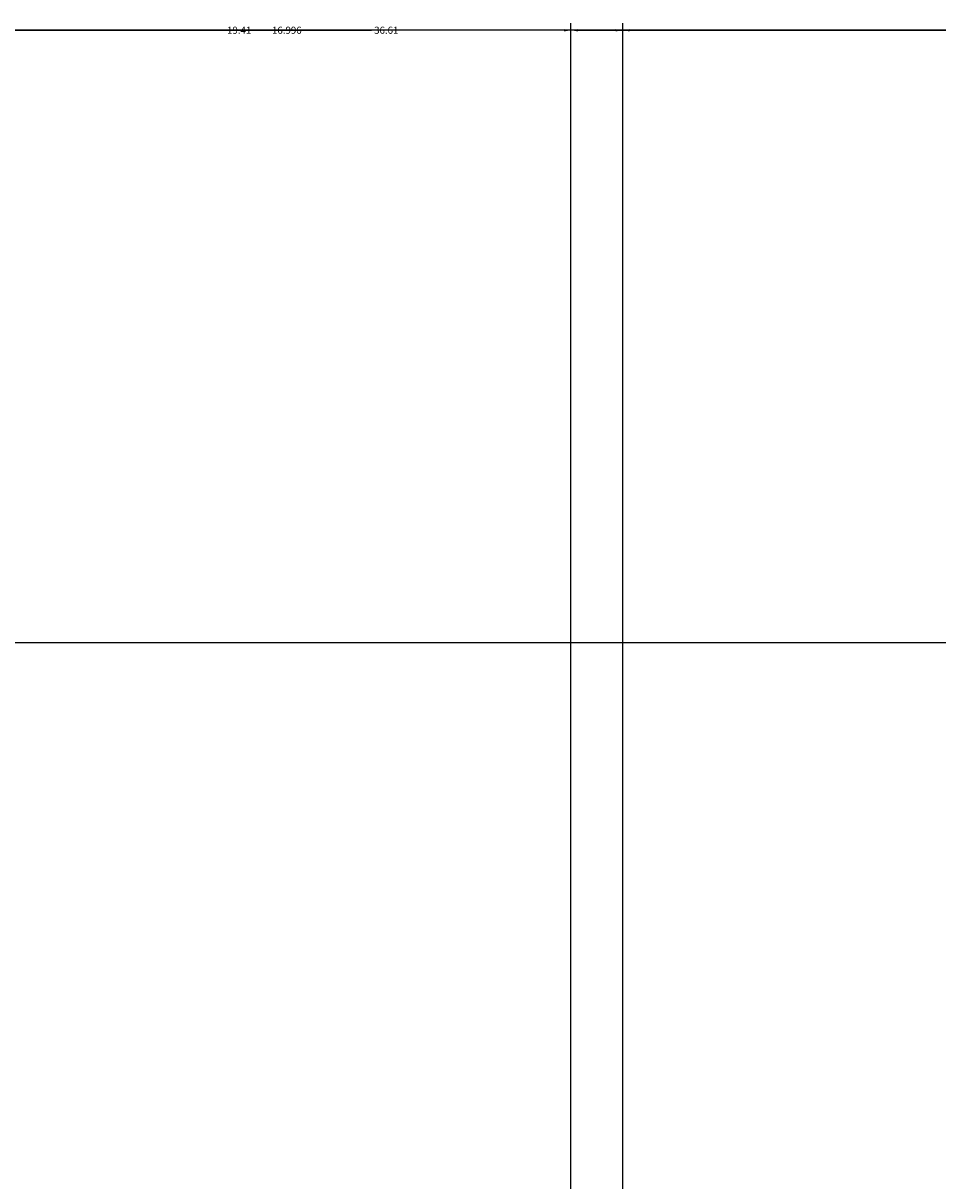
# Model space of a CAD drawing. Units: inches. Extents: x -6 to 289, y -8 to 323.
# Tile 92 of 107: x 173 to 196, y 294 to 323. Entities that reach past the tile are written whole.
import ezdxf

# ---------------------------------------------------------------- set-up
doc = ezdxf.new("R2010")
doc.units = ezdxf.units.IN
doc.header["$MEASUREMENT"] = 0
doc.layers.add('A-ANNO-DIMS', color=2, linetype='Continuous', lineweight=18)
doc.styles.get("Standard").update_dxf_attribs({"font": 'arial.ttf'})
doc.dimstyles.get("Standard").update_dxf_attribs({"dimtxt": 0.18, "dimasz": 0.18, "dimexe": 0.18, "dimexo": 0.0625, "dimgap": 0.09, "dimtad": 0, "dimtih": 1, "dimtoh": 1, "dimdec": 4, "dimzin": 0, "dimdsep": 46, "dimtxsty": 'Standard', "dimcen": 0.09, "dimadec": 0, "dimazin": 0, "dimtfac": 1, "dimtdec": 4, "dimtofl": 0, "dimtmove": 0, "dimatfit": 3, "dimfxl": 1, "dimtolj": 1, "dimtzin": 0, "dimarcsym": 0})

# ---------------------------------------------------------------- blocks, each defined once
blk = doc.blocks.new('*D12')
at = {"layer": 'A-ANNO-DIMS', "color": 0, "lineweight": -2, "transparency": 16777216}
for p, q in [((168.883, 226.717), (168.883, 322.969)), ((188.292, 226.951), (188.292, 322.969)), ((169.063, 322.789), (178.22, 322.789)), ((188.112, 322.789), (178.955, 322.789))]:
    blk.add_line(p, q, dxfattribs=at)
at = {"layer": 'A-ANNO-DIMS', "color": 0, "transparency": 16777216}
for points in [[(169.063, 322.819), (169.063, 322.759), (168.883, 322.789)], [(188.112, 322.819), (188.112, 322.759), (188.292, 322.789)]]:
    blk.add_solid(points, dxfattribs=at)
at = {"layer": 'Defpoints', "color": 0, "transparency": 16777216}
for p in [(188.292, 322.789), (188.292, 226.889), (168.883, 226.654)]:
    blk.add_point(p, dxfattribs=at)
at = {"layer": 'A-ANNO-DIMS', "color": 0, "transparency": 16777216, "insert": (178.588, 322.789), "char_height": 0.18, "attachment_point": 5}
blk.add_mtext('\\A1;19.41', dxfattribs=at)
blk = doc.blocks.new('*D13')
at = {"layer": 'A-ANNO-DIMS', "color": 0, "lineweight": -2, "transparency": 16777216}
for p, q in [((188.292, 226.951), (188.292, 322.969)), ((236.292, 226.951), (236.292, 322.969)), ((188.472, 322.789), (212.069, 322.789)), ((236.112, 322.789), (212.515, 322.789))]:
    blk.add_line(p, q, dxfattribs=at)
at = {"layer": 'A-ANNO-DIMS', "color": 0, "transparency": 16777216}
for points in [[(188.472, 322.819), (188.472, 322.759), (188.292, 322.789)], [(236.112, 322.819), (236.112, 322.759), (236.292, 322.789)]]:
    blk.add_solid(points, dxfattribs=at)
at = {"layer": 'Defpoints', "color": 0, "transparency": 16777216}
for p in [(236.292, 322.789), (188.292, 226.889), (236.292, 226.889)]:
    blk.add_point(p, dxfattribs=at)
at = {"layer": 'A-ANNO-DIMS', "color": 0, "transparency": 16777216, "insert": (212.292, 322.789), "char_height": 0.18, "attachment_point": 5}
blk.add_mtext('\\A1;48', dxfattribs=at)
blk = doc.blocks.new('*D27')
at = {"layer": 'A-ANNO-DIMS', "color": 0, "lineweight": -2, "transparency": 16777216}
for p, q in [((19.226, 307.289), (288.653, 307.289)), ((288.473, 307.109), (288.473, 277.471)), ((288.473, 247.469), (288.473, 277.107)), ((247.226, 247.289), (288.653, 247.289))]:
    blk.add_line(p, q, dxfattribs=at)
at = {"layer": 'A-ANNO-DIMS', "color": 0, "transparency": 16777216}
for points in [[(288.443, 307.109), (288.503, 307.109), (288.473, 307.289)], [(288.443, 247.469), (288.503, 247.469), (288.473, 247.289)]]:
    blk.add_solid(points, dxfattribs=at)
at = {"layer": 'Defpoints', "color": 0, "transparency": 16777216}
for p in [(19.164, 307.289), (288.473, 307.289), (247.164, 247.289)]:
    blk.add_point(p, dxfattribs=at)
at = {"layer": 'A-ANNO-DIMS', "color": 0, "transparency": 16777216, "insert": (288.473, 277.289), "char_height": 0.18, "attachment_point": 5}
blk.add_mtext('\\A1;60', dxfattribs=at)
blk = doc.blocks.new('*D79')
at = {"layer": 'A-ANNO-DIMS', "color": 0, "lineweight": -2, "transparency": 16777216}
for p, q in [((171.296, 118.033), (171.296, 322.969)), ((188.292, 116.842), (188.292, 322.969)), ((171.476, 322.789), (179.339, 322.789)), ((188.112, 322.789), (180.249, 322.789))]:
    blk.add_line(p, q, dxfattribs=at)
at = {"layer": 'A-ANNO-DIMS', "color": 0, "transparency": 16777216}
for points in [[(171.476, 322.819), (171.476, 322.759), (171.296, 322.789)], [(188.112, 322.819), (188.112, 322.759), (188.292, 322.789)]]:
    blk.add_solid(points, dxfattribs=at)
at = {"layer": 'Defpoints', "color": 0, "transparency": 16777216}
for p in [(188.292, 322.789), (171.296, 117.971), (188.292, 116.779)]:
    blk.add_point(p, dxfattribs=at)
at = {"layer": 'A-ANNO-DIMS', "color": 0, "transparency": 16777216, "insert": (179.794, 322.789), "char_height": 0.18, "attachment_point": 5}
blk.add_mtext('\\A1;16.996', dxfattribs=at)
blk = doc.blocks.new('*D80')
at = {"layer": 'A-ANNO-DIMS', "color": 0, "lineweight": -2, "transparency": 16777216}
for p, q in [((188.292, 116.842), (188.292, 322.969)), ((230.292, 116.842), (230.292, 322.969)), ((188.472, 322.789), (209.07, 322.789)), ((230.112, 322.789), (209.513, 322.789))]:
    blk.add_line(p, q, dxfattribs=at)
at = {"layer": 'A-ANNO-DIMS', "color": 0, "transparency": 16777216}
for points in [[(188.472, 322.819), (188.472, 322.759), (188.292, 322.789)], [(230.112, 322.819), (230.112, 322.759), (230.292, 322.789)]]:
    blk.add_solid(points, dxfattribs=at)
at = {"layer": 'Defpoints', "color": 0, "transparency": 16777216}
for p in [(230.292, 322.789), (188.292, 116.779), (230.292, 116.779)]:
    blk.add_point(p, dxfattribs=at)
at = {"layer": 'A-ANNO-DIMS', "color": 0, "transparency": 16777216, "insert": (209.292, 322.789), "char_height": 0.18, "attachment_point": 5}
blk.add_mtext('\\A1;42', dxfattribs=at)
blk = doc.blocks.new('*D96')
at = {"layer": 'A-ANNO-DIMS', "color": 0, "lineweight": -2, "transparency": 16777216}
for p, q in [((164.004, 159.411), (164.004, 322.969)), ((200.616, 159.411), (200.616, 322.969)), ((164.184, 322.789), (181.934, 322.789)), ((200.436, 322.789), (182.686, 322.789))]:
    blk.add_line(p, q, dxfattribs=at)
at = {"layer": 'A-ANNO-DIMS', "color": 0, "transparency": 16777216}
for points in [[(164.184, 322.819), (164.184, 322.759), (164.004, 322.789)], [(200.436, 322.819), (200.436, 322.759), (200.616, 322.789)]]:
    blk.add_solid(points, dxfattribs=at)
at = {"layer": 'Defpoints', "color": 0, "transparency": 16777216}
for p in [(200.616, 322.789), (164.004, 159.348), (200.616, 159.348)]:
    blk.add_point(p, dxfattribs=at)
at = {"layer": 'A-ANNO-DIMS', "color": 0, "transparency": 16777216, "insert": (182.31, 322.789), "char_height": 0.18, "attachment_point": 5}
blk.add_mtext('\\A1;36.61', dxfattribs=at)
blk = doc.blocks.new('*D107')
at = {"layer": 'A-ANNO-DIMS', "color": 0, "lineweight": -2, "transparency": 16777216}
for p, q in [((118.164, 293.728), (118.164, 322.969)), ((186.984, 291.541), (186.984, 322.969)), ((118.344, 322.789), (152.18, 322.789)), ((186.804, 322.789), (152.967, 322.789))]:
    blk.add_line(p, q, dxfattribs=at)
at = {"layer": 'A-ANNO-DIMS', "color": 0, "transparency": 16777216}
for points in [[(118.344, 322.819), (118.344, 322.759), (118.164, 322.789)], [(186.804, 322.819), (186.804, 322.759), (186.984, 322.789)]]:
    blk.add_solid(points, dxfattribs=at)
at = {"layer": 'Defpoints', "color": 0, "transparency": 16777216}
for p in [(186.984, 322.789), (118.164, 293.666), (186.984, 291.478)]:
    blk.add_point(p, dxfattribs=at)
at = {"layer": 'A-ANNO-DIMS', "color": 0, "transparency": 16777216, "insert": (152.574, 322.789), "char_height": 0.18, "attachment_point": 5}
blk.add_mtext('\\A1;68.82', dxfattribs=at)
blk = doc.blocks.new('*D108')
at = {"layer": 'A-ANNO-DIMS', "color": 0, "lineweight": -2, "transparency": 16777216}
for p, q in [((186.984, 291.541), (186.984, 322.969)), ((255.804, 291.541), (255.804, 322.969)), ((187.164, 322.789), (221, 322.789)), ((255.624, 322.789), (221.787, 322.789))]:
    blk.add_line(p, q, dxfattribs=at)
at = {"layer": 'A-ANNO-DIMS', "color": 0, "transparency": 16777216}
for points in [[(187.164, 322.819), (187.164, 322.759), (186.984, 322.789)], [(255.624, 322.819), (255.624, 322.759), (255.804, 322.789)]]:
    blk.add_solid(points, dxfattribs=at)
at = {"layer": 'Defpoints', "color": 0, "transparency": 16777216}
for p in [(255.804, 322.789), (186.984, 291.478), (255.804, 291.478)]:
    blk.add_point(p, dxfattribs=at)
at = {"layer": 'A-ANNO-DIMS', "color": 0, "transparency": 16777216, "insert": (221.394, 322.789), "char_height": 0.18, "attachment_point": 5}
blk.add_mtext('\\A1;68.82', dxfattribs=at)
blk = doc.blocks.new('*D118')
at = {"layer": 'A-ANNO-DIMS', "color": 0, "lineweight": -2, "transparency": 16777216}
for p, q in [((118.226, 307.289), (288.653, 307.289)), ((288.473, 307.109), (288.473, 300.659)), ((288.473, 293.846), (288.473, 300.295)), ((257.703, 293.666), (288.653, 293.666))]:
    blk.add_line(p, q, dxfattribs=at)
at = {"layer": 'A-ANNO-DIMS', "color": 0, "transparency": 16777216}
for points in [[(288.443, 307.109), (288.503, 307.109), (288.473, 307.289)], [(288.443, 293.846), (288.503, 293.846), (288.473, 293.666)]]:
    blk.add_solid(points, dxfattribs=at)
at = {"layer": 'Defpoints', "color": 0, "transparency": 16777216}
for p in [(118.164, 307.289), (288.473, 307.289), (257.641, 293.666)]:
    blk.add_point(p, dxfattribs=at)
at = {"layer": 'A-ANNO-DIMS', "color": 0, "transparency": 16777216, "insert": (288.473, 300.477), "char_height": 0.18, "attachment_point": 5}
blk.add_mtext('\\A1;13.623', dxfattribs=at)

msp = doc.modelspace()

# ---------------------------------------------------------------- dimensions: what is measured, and where the dimension line sits
at = {"layer": 'A-ANNO-DIMS'}
for base, p1, p2, override, picture, middle in [((186.9837, 322.7888), (118.1638, 293.6657), (186.9837, 291.4781), {"dimdec": 2, "dimlfac": 1, "dimrnd": 0, "dimzin": 0, "dimdsep": 46, "dimlunit": 2}, '*D107', (152.5737, 322.7888)), ((200.6162, 322.7888), (164.0039, 159.3484), (200.6162, 159.3484), {"dimdec": 2, "dimlfac": 1, "dimrnd": 0, "dimzin": 0, "dimdsep": 46, "dimlunit": 2}, '*D96', (182.3101, 322.7888)), ((188.2918, 322.7888), (168.8835, 226.654), (188.2918, 226.8887), {"dimdec": 2, "dimlfac": 1, "dimrnd": 0, "dimzin": 0, "dimdsep": 46, "dimlunit": 2}, '*D12', (178.5876, 322.7888)), ((188.2918, 322.7888), (171.296, 117.9706), (188.2918, 116.7795), {"dimdec": 3, "dimlfac": 1, "dimrnd": 0, "dimzin": 0, "dimdsep": 46, "dimlunit": 2}, '*D79', (179.7939, 322.7888)), ((255.8036, 322.7888), (186.9837, 291.4781), (255.8036, 291.4781), {"dimdec": 2, "dimlfac": 1, "dimrnd": 0, "dimzin": 0, "dimdsep": 46, "dimlunit": 2}, '*D108', (221.3936, 322.7888)), ((236.2918, 322.7888), (188.2918, 226.8887), (236.2918, 226.8887), {"dimdec": 0, "dimlfac": 1, "dimrnd": 0, "dimzin": 0, "dimdsep": 46, "dimlunit": 2}, '*D13', (212.2918, 322.7888)), ((230.2918, 322.7888), (188.2918, 116.7795), (230.2918, 116.7795), {"dimdec": 0, "dimlfac": 1, "dimrnd": 0, "dimzin": 0, "dimdsep": 46, "dimlunit": 2}, '*D80', (209.2918, 322.7888))]:
    dim = msp.add_linear_dim(base=base, p1=p1, p2=p2, dimstyle='Standard', override=override, dxfattribs=at)
    dim.commit()
    dim.dimension.update_dxf_attribs({"geometry": picture, "text_midpoint": middle})
for p1, p2, override, picture, middle in [((247.1638, 247.2888), (19.1638, 307.2888), {"dimdec": 0, "dimlfac": 1, "dimrnd": 0, "dimzin": 0, "dimdsep": 46, "dimlunit": 2}, '*D27', (288.4733, 277.2888)), ((257.6407, 293.6657), (118.1638, 307.2888), {"dimdec": 3, "dimlfac": 1, "dimrnd": 0, "dimzin": 0, "dimdsep": 46, "dimlunit": 2}, '*D118', (288.4733, 300.4773))]:
    dim = msp.add_linear_dim(base=(288.4733, 307.2888), p1=p1, p2=p2, angle=90, dimstyle='Standard', override=override, dxfattribs=at)
    dim.commit()
    dim.dimension.update_dxf_attribs({"geometry": picture, "text_midpoint": middle})

doc.saveas('drawing.dxf')
